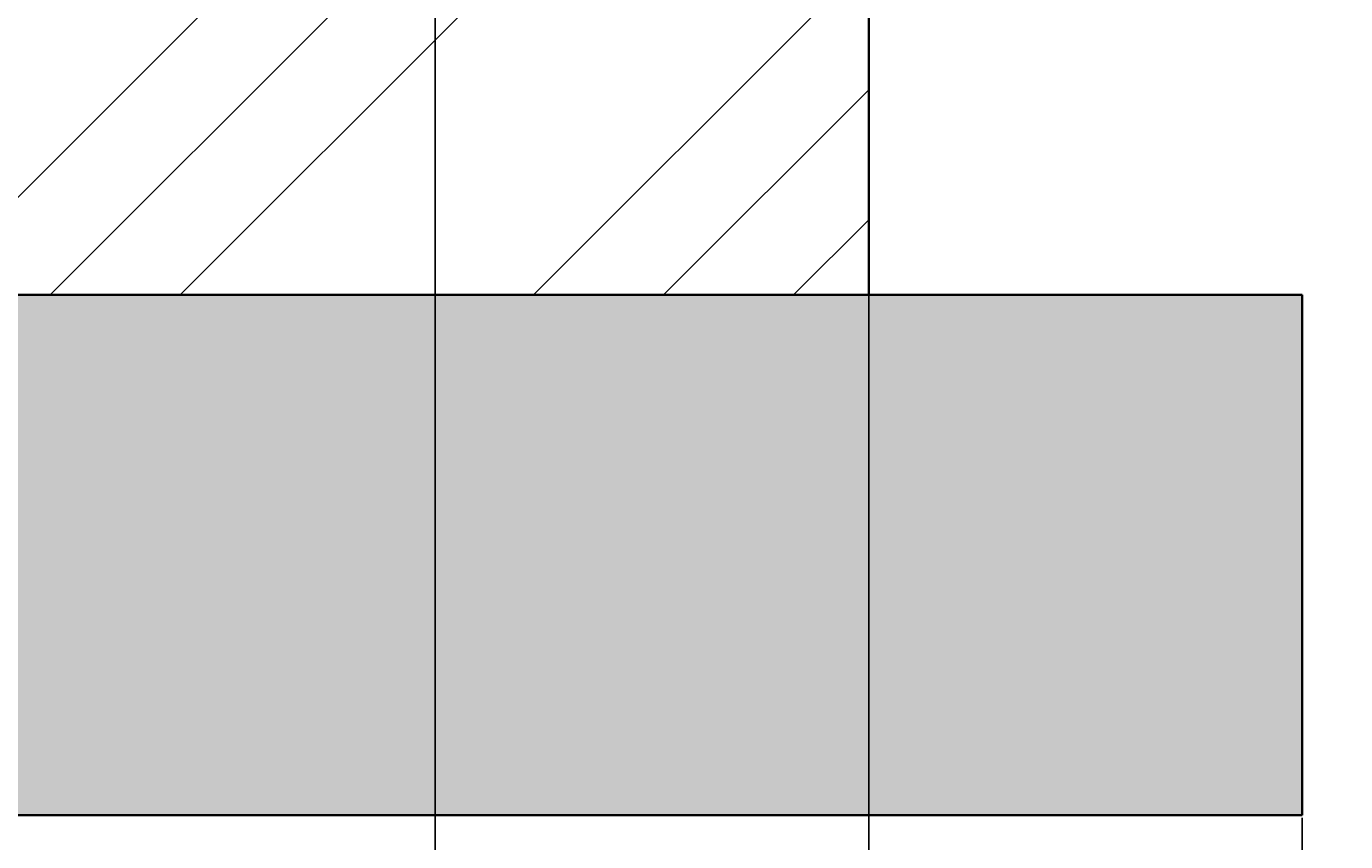
# Model space of a CAD drawing. Units: inches. Extents: x -128 to 854, y -395 to 398.
# Tile 6 of 61: x -47 to -16, y -359 to -340. Entities that reach past the tile are written whole.
import ezdxf

# ---------------------------------------------------------------- set-up
doc = ezdxf.new("R2010")
doc.units = ezdxf.units.IN
doc.header["$MEASUREMENT"] = 0
for name, color, linetype, lineweight in [('A-ANNO-DIMS', 2, 'Continuous', 18), ('A-SECT-PATT', 8, 'Continuous', 13), ('S-FNDN', 2, 'Continuous', 35), ('S-FNDN-PATT', 8, 'Continuous', 13)]:
    doc.layers.add(name, color=color, linetype=linetype, lineweight=lineweight)
doc.styles.get("Standard").update_dxf_attribs({"font": 'arial.ttf'})
doc.dimstyles.get("Standard").update_dxf_attribs({"dimtxt": 0.18, "dimasz": 0.18, "dimexe": 0.18, "dimexo": 0.0625, "dimgap": 0.09, "dimtad": 0, "dimtih": 1, "dimtoh": 1, "dimdec": 1, "dimzin": 0, "dimdsep": 46, "dimlunit": 4, "dimtxsty": 'Standard', "dimcen": 0.09, "dimclrd": 1, "dimclre": 2, "dimclrt": 6, "dimadec": 0, "dimazin": 0, "dimtfac": 1, "dimtdec": 1, "dimtofl": 0, "dimtmove": 0, "dimatfit": 3, "dimfxl": 1, "dimtfill": 2, "dimtfillclr": 3, "dimtolj": 1, "dimtzin": 0, "dimarcsym": 0})

# ---------------------------------------------------------------- blocks, each defined once
blk = doc.blocks.new('*D122')
at = {"layer": 'A-ANNO-DIMS', "color": 2, "lineweight": -2, "transparency": 16777216}
for p, q in [((-76.161, -358.082), (-76.161, -381.899)), ((-17.161, -358.082), (-17.161, -381.899))]:
    blk.add_line(p, q, dxfattribs=at)
at = {"layer": 'A-ANNO-DIMS', "color": 1, "lineweight": -2, "transparency": 16777216}
for p, q in [((-75.981, -381.719), (-47.064, -381.719)), ((-17.341, -381.719), (-46.258, -381.719))]:
    blk.add_line(p, q, dxfattribs=at)
at = {"layer": 'A-ANNO-DIMS', "color": 1, "transparency": 16777216}
for points in [[(-75.981, -381.689), (-75.981, -381.749), (-76.161, -381.719)], [(-17.341, -381.689), (-17.341, -381.749), (-17.161, -381.719)]]:
    blk.add_solid(points, dxfattribs=at)
at = {"layer": 'Defpoints', "color": 0, "transparency": 16777216}
for p in [(-76.161, -358.019), (-17.161, -358.019), (-17.161, -381.719)]:
    blk.add_point(p, dxfattribs=at)
at = {"layer": 'A-ANNO-DIMS', "color": 6, "transparency": 16777216, "insert": (-46.661, -381.719), "char_height": 0.18, "attachment_point": 5, "bg_fill": 1, "box_fill_scale": 1.25, "bg_fill_color": 3, "bg_fill_transparency": 0}
blk.add_mtext('\\A1;4\'-11"', dxfattribs=at)
blk = doc.blocks.new('*D123')
at = {"layer": 'A-ANNO-DIMS', "color": 2, "lineweight": -2, "transparency": 16777216}
for p, q in [((-17.161, -358.082), (-17.161, -381.899)), ((121.839, -358.082), (121.839, -381.899))]:
    blk.add_line(p, q, dxfattribs=at)
at = {"layer": 'A-ANNO-DIMS', "color": 1, "lineweight": -2, "transparency": 16777216}
for p, q in [((-16.981, -381.719), (51.948, -381.719)), ((121.659, -381.719), (52.73, -381.719))]:
    blk.add_line(p, q, dxfattribs=at)
at = {"layer": 'A-ANNO-DIMS', "color": 1, "transparency": 16777216}
for points in [[(-16.981, -381.689), (-16.981, -381.749), (-17.161, -381.719)], [(121.659, -381.689), (121.659, -381.749), (121.839, -381.719)]]:
    blk.add_solid(points, dxfattribs=at)
at = {"layer": 'Defpoints', "color": 0, "transparency": 16777216}
for p in [(-17.161, -358.019), (121.839, -358.019), (121.839, -381.719)]:
    blk.add_point(p, dxfattribs=at)
at = {"layer": 'A-ANNO-DIMS', "color": 6, "transparency": 16777216, "insert": (52.339, -381.719), "char_height": 0.18, "attachment_point": 5, "bg_fill": 1, "box_fill_scale": 1.25, "bg_fill_color": 3, "bg_fill_transparency": 0}
blk.add_mtext('\\A1;11\'-7"', dxfattribs=at)
blk = doc.blocks.new('*D125')
at = {"layer": 'A-ANNO-DIMS', "color": 2, "lineweight": -2, "transparency": 16777216}
for p, q in [((-37.161, -298.082), (-37.161, -381.899)), ((22.811, -298.082), (22.811, -381.899))]:
    blk.add_line(p, q, dxfattribs=at)
at = {"layer": 'A-ANNO-DIMS', "color": 1, "lineweight": -2, "transparency": 16777216}
for p, q in [((-36.981, -381.719), (-7.504, -381.719)), ((22.631, -381.719), (-6.846, -381.719))]:
    blk.add_line(p, q, dxfattribs=at)
at = {"layer": 'A-ANNO-DIMS', "color": 1, "transparency": 16777216}
for points in [[(-36.981, -381.689), (-36.981, -381.749), (-37.161, -381.719)], [(22.631, -381.689), (22.631, -381.749), (22.811, -381.719)]]:
    blk.add_solid(points, dxfattribs=at)
at = {"layer": 'Defpoints', "color": 0, "transparency": 16777216}
for p in [(-37.161, -298.019), (22.811, -298.019), (22.811, -381.719)]:
    blk.add_point(p, dxfattribs=at)
at = {"layer": 'A-ANNO-DIMS', "color": 6, "transparency": 16777216, "insert": (-7.175, -381.719), "char_height": 0.18, "attachment_point": 5, "bg_fill": 1, "box_fill_scale": 1.25, "bg_fill_color": 3, "bg_fill_transparency": 0}
blk.add_mtext('\\A1;5\'-0"', dxfattribs=at)
blk = doc.blocks.new('*D128')
at = {"layer": 'A-ANNO-DIMS', "color": 2, "lineweight": -2, "transparency": 16777216}
for p, q in [((-17.223, -346.019), (-128.041, -346.019)), ((-17.223, -358.019), (-128.041, -358.019))]:
    blk.add_line(p, q, dxfattribs=at)
at = {"layer": 'A-ANNO-DIMS', "color": 1, "lineweight": -2, "transparency": 16777216}
for p, q in [((-127.861, -346.199), (-127.861, -351.837)), ((-127.861, -357.839), (-127.861, -352.201))]:
    blk.add_line(p, q, dxfattribs=at)
at = {"layer": 'A-ANNO-DIMS', "color": 1, "transparency": 16777216}
for points in [[(-127.891, -346.199), (-127.831, -346.199), (-127.861, -346.019)], [(-127.891, -357.839), (-127.831, -357.839), (-127.861, -358.019)]]:
    blk.add_solid(points, dxfattribs=at)
at = {"layer": 'Defpoints', "color": 0, "transparency": 16777216}
for p in [(-127.861, -346.019), (-17.161, -346.019), (-17.161, -358.019)]:
    blk.add_point(p, dxfattribs=at)
at = {"layer": 'A-ANNO-DIMS', "color": 6, "transparency": 16777216, "insert": (-127.861, -352.019), "char_height": 0.18, "attachment_point": 5, "bg_fill": 1, "box_fill_scale": 1.25, "bg_fill_color": 3, "bg_fill_transparency": 0}
blk.add_mtext('\\A1;1\'-0"', dxfattribs=at)
blk = doc.blocks.new('*D129')
at = {"layer": 'A-ANNO-DIMS', "color": 2, "lineweight": -2, "transparency": 16777216}
for p, q in [((-27.223, -322.019), (-128.041, -322.019)), ((-27.223, -346.019), (-128.041, -346.019))]:
    blk.add_line(p, q, dxfattribs=at)
at = {"layer": 'A-ANNO-DIMS', "color": 1, "lineweight": -2, "transparency": 16777216}
for p, q in [((-127.861, -322.199), (-127.861, -333.837)), ((-127.861, -345.839), (-127.861, -334.201))]:
    blk.add_line(p, q, dxfattribs=at)
at = {"layer": 'A-ANNO-DIMS', "color": 1, "transparency": 16777216}
for points in [[(-127.891, -322.199), (-127.831, -322.199), (-127.861, -322.019)], [(-127.891, -345.839), (-127.831, -345.839), (-127.861, -346.019)]]:
    blk.add_solid(points, dxfattribs=at)
at = {"layer": 'Defpoints', "color": 0, "transparency": 16777216}
for p in [(-127.861, -322.019), (-27.161, -322.019), (-27.161, -346.019)]:
    blk.add_point(p, dxfattribs=at)
at = {"layer": 'A-ANNO-DIMS', "color": 6, "transparency": 16777216, "insert": (-127.861, -334.019), "char_height": 0.18, "attachment_point": 5, "bg_fill": 1, "box_fill_scale": 1.25, "bg_fill_color": 3, "bg_fill_transparency": 0}
blk.add_mtext('\\A1;2\'-0"', dxfattribs=at)
blk = doc.blocks.new('*D130')
at = {"layer": 'A-ANNO-DIMS', "color": 2, "lineweight": -2, "transparency": 16777216}
for p, q in [((-66.161, -322.082), (-66.161, -381.899)), ((-27.161, -322.082), (-27.161, -381.899))]:
    blk.add_line(p, q, dxfattribs=at)
at = {"layer": 'A-ANNO-DIMS', "color": 1, "lineweight": -2, "transparency": 16777216}
for p, q in [((-65.981, -381.719), (-46.99, -381.719)), ((-27.341, -381.719), (-46.332, -381.719))]:
    blk.add_line(p, q, dxfattribs=at)
at = {"layer": 'A-ANNO-DIMS', "color": 1, "transparency": 16777216}
for points in [[(-65.981, -381.689), (-65.981, -381.749), (-66.161, -381.719)], [(-27.341, -381.689), (-27.341, -381.749), (-27.161, -381.719)]]:
    blk.add_solid(points, dxfattribs=at)
at = {"layer": 'Defpoints', "color": 0, "transparency": 16777216}
for p in [(-66.161, -322.019), (-27.161, -322.019), (-27.161, -381.719)]:
    blk.add_point(p, dxfattribs=at)
at = {"layer": 'A-ANNO-DIMS', "color": 6, "transparency": 16777216, "insert": (-46.661, -381.719), "char_height": 0.18, "attachment_point": 5, "bg_fill": 1, "box_fill_scale": 1.25, "bg_fill_color": 3, "bg_fill_transparency": 0}
blk.add_mtext('\\A1;3\'-3"', dxfattribs=at)

msp = doc.modelspace()

# ---------------------------------------------------------------- hatches: boundary and pattern name
at = {"layer": 'A-SECT-PATT'}
h = msp.add_hatch(dxfattribs=at)
h.set_pattern_fill('GOST_GROUND', color=256)
h.set_pattern_definition([(45, (0, 0), (14.14214, -9e-16), [20]), (45, (3, 0), (14.14214, -9e-16), [20]), (45, (6, 0), (14.14214, -9e-16), [20])])
h.paths.add_polyline_path([(-27.161, -322.019), (-37.161, -322.019), (-37.161, -298.019), (-56.161, -298.019), (-56.161, -322.019), (-66.161, -322.019), (-66.161, -346.019), (-27.161, -346.019)])
h.paths.add_polyline_path([(170.839, -322.019), (160.839, -322.019), (160.839, -298.019), (155.839, -298.019), (141.839, -298.019), (141.839, -322.019), (131.839, -322.019), (131.839, -346.019), (170.839, -346.019)])
h.paths.add_polyline_path([(327.839, -322.019), (317.839, -322.019), (317.839, -298.019), (312.839, -298.019), (298.839, -298.019), (298.839, -322.019), (288.839, -322.019), (288.839, -346.019), (327.839, -346.019)])
h.paths.add_polyline_path([(-37.161, -274.019), (-56.161, -274.019), (-56.161, -298.019), (-37.161, -298.019)])
h.paths.add_polyline_path([(-37.161, -207.019), (-56.161, -207.019), (-56.161, -226.019), (-37.161, -226.019)])
h.paths.add_polyline_path([(160.839, -274.019), (141.839, -274.019), (141.839, -298.019), (155.839, -298.019), (160.839, -298.019)])
at = {"layer": 'S-FNDN-PATT'}
h = msp.add_hatch(dxfattribs=at)
h.set_pattern_fill('AR-CONC', color=256)
h.paths.add_polyline_path([(-17.161, -346.019), (-27.161, -346.019), (-66.161, -346.019), (-76.161, -346.019), (-76.161, -358.019), (-17.161, -358.019)])
h.paths.add_polyline_path([(180.839, -346.019), (170.839, -346.019), (131.839, -346.019), (121.839, -346.019), (121.839, -358.019), (180.839, -358.019)])
h.paths.add_polyline_path([(337.839, -346.019), (327.839, -346.019), (288.839, -346.019), (278.839, -346.019), (278.839, -358.019), (337.839, -358.019)])

# ---------------------------------------------------------------- linework, layer by layer
at = {"layer": 'S-FNDN'}
for p, q in [((-27.161, -322.019), (-27.161, -346.019)), ((-66.161, -346.019), (-27.161, -346.019)), ((-27.161, -346.019), (-17.161, -346.019)), ((-17.161, -346.019), (-17.161, -358.019)), ((-76.161, -358.019), (-17.161, -358.019))]:
    msp.add_line(p, q, dxfattribs=at)

# ---------------------------------------------------------------- dimensions: what is measured, and where the dimension line sits
at = {"layer": 'A-ANNO-DIMS'}
for base, p1, p2, picture, middle in [((22.811, -381.719), (-37.161, -298.019), (22.811, -298.019), '*D125', (-7.175, -381.719)), ((-27.161, -381.719), (-66.161, -322.019), (-27.161, -322.019), '*D130', (-46.661, -381.719)), ((-17.161, -381.719), (-76.161, -358.019), (-17.161, -358.019), '*D122', (-46.661, -381.719)), ((121.839, -381.719), (-17.161, -358.019), (121.839, -358.019), '*D123', (52.339, -381.719))]:
    dim = msp.add_linear_dim(base=base, p1=p1, p2=p2, dimstyle='Standard', override={"dimdec": 1, "dimlfac": 1, "dimrnd": 0, "dimzin": 1, "dimdsep": 46, "dimlunit": 4, "dimfrac": 2}, dxfattribs=at)
    dim.commit()
    dim.dimension.update_dxf_attribs({"geometry": picture, "text_midpoint": middle})
for base, p1, p2, picture, middle in [((-127.861, -322.019), (-27.161, -346.019), (-27.161, -322.019), '*D129', (-127.861, -334.019)), ((-127.861, -346.019), (-17.161, -358.019), (-17.161, -346.019), '*D128', (-127.861, -352.019))]:
    dim = msp.add_linear_dim(base=base, p1=p1, p2=p2, angle=90, dimstyle='Standard', override={"dimdec": 1, "dimlfac": 1, "dimrnd": 0, "dimzin": 1, "dimdsep": 46, "dimlunit": 4, "dimfrac": 2}, dxfattribs=at)
    dim.commit()
    dim.dimension.update_dxf_attribs({"geometry": picture, "text_midpoint": middle})

doc.saveas('drawing.dxf')
